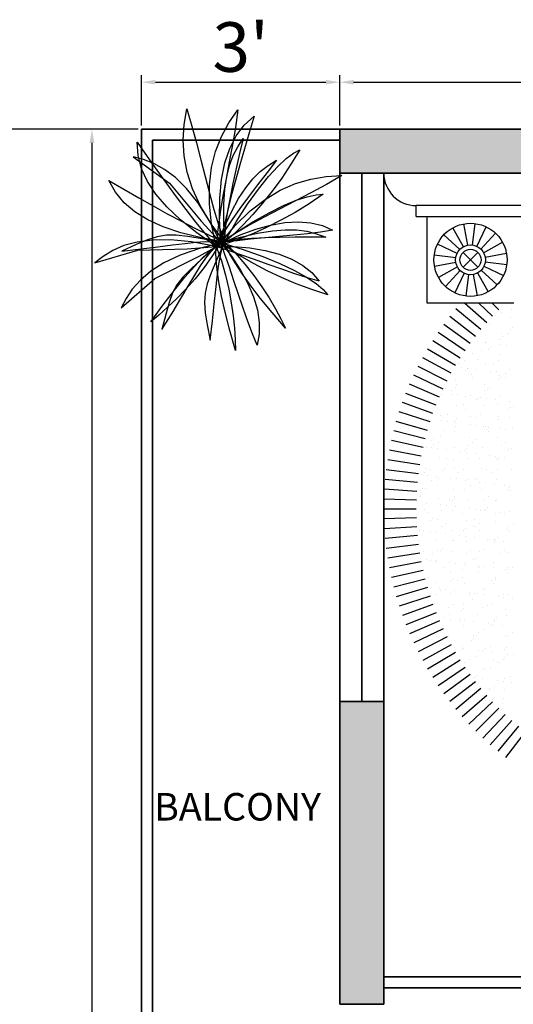
# Model space of a CAD drawing. Units: inches. Extents: x 1566 to 2546, y 1087 to 2705.
# Tile 20 of 27: x 2040 to 2130, y 1625 to 1804. Entities that reach past the tile are written whole.
import ezdxf

# ---------------------------------------------------------------- set-up
doc = ezdxf.new("R2010")
doc.units = ezdxf.units.IN
for name, color, linetype, lineweight in [('A-ANNO-DIMS', 2, 'Continuous', 18), ('A-AREA-IDEN', 7, 'Continuous', 18), ('A-FURN', 8, 'Continuous', 18), ('A-WALL', 7, 'Continuous', 35), ('A-WALL-PATT', 8, 'Continuous', 13), ('L-PLNT', 94, 'Continuous', 18)]:
    doc.layers.add(name, color=color, linetype=linetype, lineweight=lineweight)
for name, color, linetype in [('A-FRN', 11, 'Continuous'), ('A-HT', 15, 'Continuous'), ('DIENHOA', 3, 'Continuous'), ('L-HT', 1, 'Continuous')]:
    doc.layers.add(name, color=color, linetype=linetype)
doc.styles.get("Standard").update_dxf_attribs({"font": 'arial.ttf'})
doc.dimstyles.new('ISO-25', dxfattribs={"dimtxt": 2.5, "dimasz": 2.5, "dimexe": 1.25, "dimexo": 0.625, "dimtad": 1, "dimtxsty": 'Standard', "dimcen": 2.5, "dimadec": 0, "dimazin": 0, "dimtfac": 1, "dimtmove": 0, "dimatfit": 3, "dimfxl": 1, "dimarcsym": 0})

# ---------------------------------------------------------------- blocks, each defined once
blk = doc.blocks.new('*D1')
at = {"layer": 'A-ANNO-DIMS', "color": 0, "lineweight": -2, "transparency": 16777216}
for p, q in [((2062.29, 1785.06), (2062.29, 1794.2)), ((2098.29, 1785.06), (2098.29, 1794.2)), ((2064.79, 1792.95), (2095.79, 1792.95))]:
    blk.add_line(p, q, dxfattribs=at)
at = {"layer": 'A-ANNO-DIMS', "color": 0, "transparency": 16777216}
for points in [[(2064.79, 1793.37), (2064.79, 1792.53), (2062.29, 1792.95)], [(2095.79, 1793.37), (2095.79, 1792.53), (2098.29, 1792.95)]]:
    blk.add_solid(points, dxfattribs=at)
at = {"layer": 'Defpoints', "color": 0, "transparency": 16777216}
for p in [(2098.29, 1792.95), (2062.29, 1784.43), (2098.29, 1784.43)]:
    blk.add_point(p, dxfattribs=at)
at = {"layer": 'A-ANNO-DIMS', "color": 0, "transparency": 16777216, "insert": (2080.29, 1798.17), "char_height": 9, "attachment_point": 5}
blk.add_mtext("3'", dxfattribs=at)
blk = doc.blocks.new('*D2')
at = {"layer": 'A-ANNO-DIMS', "color": 0, "lineweight": -2, "transparency": 16777216}
for p, q in [((2098.29, 1785.06), (2098.29, 1794.2)), ((2458.29, 1785.06), (2458.29, 1794.2)), ((2100.79, 1792.95), (2455.79, 1792.95))]:
    blk.add_line(p, q, dxfattribs=at)
at = {"layer": 'A-ANNO-DIMS', "color": 0, "transparency": 16777216}
for points in [[(2100.79, 1793.37), (2100.79, 1792.53), (2098.29, 1792.95)], [(2455.79, 1793.37), (2455.79, 1792.53), (2458.29, 1792.95)]]:
    blk.add_solid(points, dxfattribs=at)
at = {"layer": 'Defpoints', "color": 0, "transparency": 16777216}
for p in [(2458.29, 1792.95), (2098.29, 1784.43), (2458.29, 1784.43)]:
    blk.add_point(p, dxfattribs=at)
at = {"layer": 'A-ANNO-DIMS', "color": 0, "transparency": 16777216, "insert": (2278.29, 1798.17), "char_height": 9, "attachment_point": 5}
blk.add_mtext("30'", dxfattribs=at)
blk = doc.blocks.new('*D3')
at = {"layer": 'A-ANNO-DIMS', "color": 0, "lineweight": -2, "transparency": 16777216}
for p, q in [((2061.66, 1784.43), (2052.02, 1784.43)), ((2053.27, 1781.93), (2053.27, 1162.93)), ((2061.66, 1160.43), (2052.02, 1160.43))]:
    blk.add_line(p, q, dxfattribs=at)
at = {"layer": 'A-ANNO-DIMS', "color": 0, "transparency": 16777216}
for points in [[(2052.85, 1781.93), (2053.69, 1781.93), (2053.27, 1784.43)], [(2052.85, 1162.93), (2053.69, 1162.93), (2053.27, 1160.43)]]:
    blk.add_solid(points, dxfattribs=at)
at = {"layer": 'Defpoints', "color": 0, "transparency": 16777216}
for p in [(2062.29, 1784.43), (2053.27, 1160.43), (2062.29, 1160.43)]:
    blk.add_point(p, dxfattribs=at)
at = {"layer": 'A-ANNO-DIMS', "color": 0, "transparency": 16777216, "insert": (2048.05, 1472.43), "char_height": 9, "attachment_point": 5, "rotation": 90}
blk.add_mtext("52'", dxfattribs=at)
blk = doc.blocks.new('*X21')
at = {"color": 0}
for p, q in [((1.0951, 2.4744), (1.0951, 2.4744)), ((1.0521, 2.4302), (1.0521, 2.4302)), ((1.0613, 2.4218), (1.0613, 2.4218)), ((1.0963, 2.4457), (1.0963, 2.4457)), ((1.1027, 2.4263), (1.1027, 2.4263)), ((1.0383, 2.3768), (1.0383, 2.3768)), ((1.0397, 2.3823), (1.0397, 2.3823)), ((1.0608, 2.3689), (1.0608, 2.3689)), ((1.1048, 2.3819), (1.1048, 2.3819)), ((0.966, 2.3279), (0.966, 2.3279)), ((0.9708, 2.3251), (0.9708, 2.3251)), ((0.981, 2.3202), (0.981, 2.3202)), ((1.0066, 2.3333), (1.0066, 2.3333)), ((1.0745, 2.3422), (1.0745, 2.3422)), ((1.1005, 2.3457), (1.1005, 2.3457)), ((1.1059, 2.33), (1.1059, 2.33)), ((1.1367, 2.3205), (1.1367, 2.3205)), ((1.1412, 2.351), (1.1412, 2.351)), ((1.0043, 2.2924), (1.0043, 2.2924)), ((1.0135, 2.284), (1.0135, 2.284)), ((1.0414, 2.2805), (1.0414, 2.2805)), ((0.9244, 2.2568), (0.9244, 2.2568)), ((0.9455, 2.2434), (0.9455, 2.2434)), ((0.974, 2.2287), (0.974, 2.2287)), ((1.057, 2.2441), (1.057, 2.2441)), ((1.0801, 2.2571), (1.0801, 2.2571)), ((1.1012, 2.2437), (1.1012, 2.2437)), ((1.109, 2.2336), (1.109, 2.2336)), ((0.8775, 2.1868), (0.8775, 2.1868)), ((0.9067, 2.2002), (0.9067, 2.2002)), ((0.9137, 2.1825), (0.9137, 2.1825)), ((0.9181, 2.1922), (0.9181, 2.1922)), ((0.986, 2.2011), (0.986, 2.2011)), ((1.0121, 2.2046), (1.0121, 2.2046)), ((1.0214, 2.195), (1.0214, 2.195)), ((1.0446, 2.1841), (1.0446, 2.1841)), ((1.0527, 2.2099), (1.0527, 2.2099)), ((1.1068, 2.1985), (1.1068, 2.1985)), ((1.116, 2.1901), (1.116, 2.1901)), ((1.1206, 2.2189), (1.1206, 2.2189)), ((1.1466, 2.2223), (1.1466, 2.2223)), ((0.9565, 2.1546), (0.9565, 2.1546)), ((0.9657, 2.1462), (0.9657, 2.1462)), ((1.1122, 2.1373), (1.1122, 2.1373)), ((0.8492, 2.133), (0.8492, 2.133)), ((0.9648, 2.1316), (0.9648, 2.1316)), ((0.9771, 2.1324), (0.9771, 2.1324)), ((0.9859, 2.1182), (0.9859, 2.1182)), ((1.0092, 2.1063), (1.0092, 2.1063)), ((1.1205, 2.1319), (1.1205, 2.1319)), ((1.1416, 2.1184), (1.1416, 2.1184)), ((0.8296, 2.0511), (0.8296, 2.0511)), ((0.8589, 2.0624), (0.8589, 2.0624)), ((0.8975, 2.06), (0.8975, 2.06)), ((0.9061, 2.0695), (0.9061, 2.0695)), ((0.9169, 2.0861), (0.9169, 2.0861)), ((0.9236, 2.0635), (0.9236, 2.0635)), ((0.9642, 2.0688), (0.9642, 2.0688)), ((1.0321, 2.0777), (1.0321, 2.0777)), ((1.0477, 2.0878), (1.0477, 2.0878)), ((1.0582, 2.0812), (1.0582, 2.0812)), ((1.059, 2.0607), (1.059, 2.0607)), ((1.0618, 2.0698), (1.0618, 2.0698)), ((1.0682, 2.0523), (1.0682, 2.0523)), ((1.0988, 2.0865), (1.0988, 2.0865)), ((0.8495, 2.0061), (0.8495, 2.0061)), ((0.8524, 2.0367), (0.8524, 2.0367)), ((0.9087, 2.0168), (0.9087, 2.0168)), ((0.9179, 2.0084), (0.9179, 2.0084)), ((0.9803, 2.0361), (0.9803, 2.0361)), ((1.0052, 2.0064), (1.0052, 2.0064)), ((1.1117, 2.0124), (1.1117, 2.0124)), ((1.1153, 2.0409), (1.1153, 2.0409)), ((0.785, 1.9849), (0.785, 1.9849)), ((0.8706, 1.9927), (0.8706, 1.9927)), ((0.92, 1.9898), (0.92, 1.9898)), ((0.9614, 1.9685), (0.9614, 1.9685)), ((1.0263, 1.993), (1.0263, 1.993)), ((1.0509, 1.9915), (1.0509, 1.9915)), ((1.0782, 1.9544), (1.0782, 1.9544)), ((1.1043, 1.9578), (1.1043, 1.9578)), ((1.1449, 1.9631), (1.1449, 1.9631)), ((0.7908, 1.944), (0.7908, 1.944)), ((0.8091, 1.9189), (0.8091, 1.9189)), ((0.8111, 1.9247), (0.8111, 1.9247)), ((0.8351, 1.9223), (0.8351, 1.9223)), ((0.8555, 1.9403), (0.8555, 1.9403)), ((0.8757, 1.9277), (0.8757, 1.9277)), ((0.9436, 1.9366), (0.9436, 1.9366)), ((0.9465, 1.9443), (0.9465, 1.9443)), ((0.9697, 1.9401), (0.9697, 1.9401)), ((0.9834, 1.9397), (0.9834, 1.9397)), ((1.0103, 1.9454), (1.0103, 1.9454)), ((1.0111, 1.9229), (1.0111, 1.9229)), ((1.0204, 1.9145), (1.0204, 1.9145)), ((1.1022, 1.9446), (1.1022, 1.9446)), ((1.1185, 1.9446), (1.1185, 1.9446)), ((0.7552, 1.8672), (0.7552, 1.8672)), ((0.7881, 1.8886), (0.7881, 1.8886)), ((0.8608, 1.879), (0.8608, 1.879)), ((0.8701, 1.8706), (0.8701, 1.8706)), ((0.8898, 1.8809), (0.8898, 1.8809)), ((0.9109, 1.8675), (0.9109, 1.8675)), ((0.9232, 1.8935), (0.9232, 1.8935)), ((1.0456, 1.8812), (1.0456, 1.8812)), ((1.054, 1.8951), (1.054, 1.8951)), ((1.0639, 1.8746), (1.0639, 1.8746)), ((1.0666, 1.8678), (1.0666, 1.8678)), ((0.8311, 1.8188), (0.8311, 1.8188)), ((0.8587, 1.844), (0.8587, 1.844)), ((0.9136, 1.8307), (0.9136, 1.8307)), ((0.9866, 1.8434), (0.9866, 1.8434)), ((0.9868, 1.8191), (0.9868, 1.8191)), ((1.0564, 1.822), (1.0564, 1.822)), ((1.1136, 1.829), (1.1136, 1.829)), ((1.1216, 1.8482), (1.1216, 1.8482)), ((1.1228, 1.8206), (1.1228, 1.8206)), ((1.1243, 1.831), (1.1243, 1.831)), ((1.1425, 1.8194), (1.1425, 1.8194)), ((0.7206, 1.7778), (0.7206, 1.7778)), ((0.7466, 1.7812), (0.7466, 1.7812)), ((0.7632, 1.7869), (0.7632, 1.7869)), ((0.7872, 1.7866), (0.7872, 1.7866)), ((0.7913, 1.7922), (0.7913, 1.7922)), ((0.8552, 1.7955), (0.8552, 1.7955)), ((0.8812, 1.799), (0.8812, 1.799)), ((0.9218, 1.8043), (0.9218, 1.8043)), ((0.9263, 1.7971), (0.9263, 1.7971)), ((0.9633, 1.7851), (0.9633, 1.7851)), ((0.9725, 1.7767), (0.9725, 1.7767)), ((0.9897, 1.8132), (0.9897, 1.8132)), ((1.0158, 1.8167), (1.0158, 1.8167)), ((1.0572, 1.7988), (1.0572, 1.7988)), ((0.731, 1.746), (0.731, 1.746)), ((0.7745, 1.7554), (0.7745, 1.7554)), ((0.7956, 1.742), (0.7956, 1.742)), ((0.813, 1.7413), (0.813, 1.7413)), ((0.8222, 1.7328), (0.8222, 1.7328)), ((0.8618, 1.7477), (0.8618, 1.7477)), ((0.9302, 1.7557), (0.9302, 1.7557)), ((0.9513, 1.7423), (0.9513, 1.7423)), ((0.9897, 1.747), (0.9897, 1.747)), ((1.016, 1.7368), (1.016, 1.7368)), ((1.0859, 1.756), (1.0859, 1.756)), ((1.107, 1.7426), (1.107, 1.7426)), ((1.1248, 1.7519), (1.1248, 1.7519)), ((0.7158, 1.6933), (0.7158, 1.6933)), ((0.7944, 1.6959), (0.7944, 1.6959)), ((0.8657, 1.693), (0.8657, 1.693)), ((0.8715, 1.6936), (0.8715, 1.6936)), ((0.9295, 1.7008), (0.9295, 1.7008)), ((1.0272, 1.6939), (1.0272, 1.6939)), ((1.0358, 1.6899), (1.0358, 1.6899)), ((1.0603, 1.7024), (1.0603, 1.7024)), ((1.0619, 1.6933), (1.0619, 1.6933)), ((1.0658, 1.6912), (1.0658, 1.6912)), ((1.075, 1.6828), (1.075, 1.6828)), ((1.1025, 1.6986), (1.1025, 1.6986)), ((0.7154, 1.6491), (0.7154, 1.6491)), ((0.7341, 1.6496), (0.7341, 1.6496)), ((0.7667, 1.6544), (0.7667, 1.6544)), ((0.7927, 1.6578), (0.7927, 1.6578)), ((0.8333, 1.6632), (0.8333, 1.6632)), ((0.865, 1.6513), (0.865, 1.6513)), ((0.9013, 1.6721), (0.9013, 1.6721)), ((0.9155, 1.6474), (0.9155, 1.6474)), ((0.9247, 1.6389), (0.9247, 1.6389)), ((0.9273, 1.6756), (0.9273, 1.6756)), ((0.9679, 1.6809), (0.9679, 1.6809)), ((0.9929, 1.6507), (0.9929, 1.6507)), ((1.1185, 1.6429), (1.1185, 1.6429)), ((1.1279, 1.6556), (1.1279, 1.6556)), ((0.7652, 1.6035), (0.7652, 1.6035)), ((0.7744, 1.595), (0.7744, 1.595)), ((0.7976, 1.5996), (0.7976, 1.5996)), ((0.8149, 1.6302), (0.8149, 1.6302)), ((0.836, 1.6168), (0.836, 1.6168)), ((0.9326, 1.6044), (0.9326, 1.6044)), ((0.9682, 1.599), (0.9682, 1.599)), ((0.9706, 1.6305), (0.9706, 1.6305)), ((0.9917, 1.6171), (0.9917, 1.6171)), ((1.0635, 1.6061), (1.0635, 1.6061)), ((1.1263, 1.6308), (1.1263, 1.6308)), ((1.1474, 1.6173), (1.1474, 1.6173)), ((0.7373, 1.5533), (0.7373, 1.5533)), ((0.7562, 1.5681), (0.7562, 1.5681)), ((0.8179, 1.5552), (0.8179, 1.5552)), ((0.8681, 1.555), (0.8681, 1.555)), ((0.9119, 1.5684), (0.9119, 1.5684)), ((0.9474, 1.5488), (0.9474, 1.5488)), ((0.9734, 1.5522), (0.9734, 1.5522)), ((0.996, 1.5544), (0.996, 1.5544)), ((1.014, 1.5575), (1.014, 1.5575)), ((1.018, 1.5534), (1.018, 1.5534)), ((1.0272, 1.545), (1.0272, 1.545)), ((1.0676, 1.5687), (1.0676, 1.5687)), ((1.0819, 1.5665), (1.0819, 1.5665)), ((1.108, 1.5699), (1.108, 1.5699)), ((1.1311, 1.5592), (1.1311, 1.5592)), ((0.7042, 1.5167), (0.7042, 1.5167)), ((0.7448, 1.5221), (0.7448, 1.5221)), ((0.8007, 1.5032), (0.8007, 1.5032)), ((0.8128, 1.531), (0.8128, 1.531)), ((0.8388, 1.5345), (0.8388, 1.5345)), ((0.8553, 1.505), (0.8553, 1.505)), ((0.8677, 1.5096), (0.8677, 1.5096)), ((0.8769, 1.5011), (0.8769, 1.5011)), ((0.8794, 1.5398), (0.8794, 1.5398)), ((0.9358, 1.5081), (0.9358, 1.5081)), ((1.011, 1.5053), (1.011, 1.5053)), ((1.0666, 1.5098), (1.0666, 1.5098)), ((1.0707, 1.5051), (1.0707, 1.5051)), ((0.7174, 1.4657), (0.7174, 1.4657)), ((0.7207, 1.4913), (0.7207, 1.4913)), ((0.7266, 1.4572), (0.7266, 1.4572)), ((0.7404, 1.457), (0.7404, 1.457)), ((0.8713, 1.4586), (0.8713, 1.4586)), ((0.8764, 1.4916), (0.8764, 1.4916)), ((0.9204, 1.4613), (0.9204, 1.4613)), ((0.9992, 1.458), (0.9992, 1.458)), ((1.0321, 1.4919), (1.0321, 1.4919)), ((1.1205, 1.4595), (1.1205, 1.4595)), ((1.1342, 1.4629), (1.1342, 1.4629)), ((0.7701, 1.4174), (0.7701, 1.4174)), ((0.7966, 1.4429), (0.7966, 1.4429)), ((0.8849, 1.4111), (0.8849, 1.4111)), ((0.9255, 1.4164), (0.9255, 1.4164)), ((0.9389, 1.4118), (0.9389, 1.4118)), ((0.9523, 1.4432), (0.9523, 1.4432)), ((0.9701, 1.4157), (0.9701, 1.4157)), ((0.9935, 1.4254), (0.9935, 1.4254)), ((1.0195, 1.4288), (1.0195, 1.4288)), ((1.0601, 1.4341), (1.0601, 1.4341)), ((1.0698, 1.4134), (1.0698, 1.4134)), ((1.108, 1.4435), (1.108, 1.4435)), ((1.128, 1.4431), (1.128, 1.4431)), ((1.1297, 1.4511), (1.1297, 1.4511)), ((0.7243, 1.3899), (0.7243, 1.3899)), ((0.74, 1.3795), (0.74, 1.3795)), ((0.7503, 1.3934), (0.7503, 1.3934)), ((0.761, 1.3661), (0.761, 1.3661)), ((0.7909, 1.3987), (0.7909, 1.3987)), ((0.8039, 1.4069), (0.8039, 1.4069)), ((0.8198, 1.3718), (0.8198, 1.3718)), ((0.8291, 1.3633), (0.8291, 1.3633)), ((0.8589, 1.4076), (0.8589, 1.4076)), ((0.8957, 1.3798), (0.8957, 1.3798)), ((0.9168, 1.3664), (0.9168, 1.3664)), ((0.9794, 1.4072), (0.9794, 1.4072)), ((1.0229, 1.3673), (1.0229, 1.3673)), ((1.0514, 1.3801), (1.0514, 1.3801)), ((1.0725, 1.3667), (1.0725, 1.3667)), ((1.1374, 1.3665), (1.1374, 1.3665)), ((0.7436, 1.3606), (0.7436, 1.3606)), ((0.837, 1.3177), (0.837, 1.3177)), ((0.8726, 1.3235), (0.8726, 1.3235)), ((0.8744, 1.3623), (0.8744, 1.3623)), ((0.9927, 1.318), (0.9927, 1.318)), ((1.0023, 1.3617), (1.0023, 1.3617)), ((1.0726, 1.3217), (1.0726, 1.3217)), ((0.807, 1.3105), (0.807, 1.3105)), ((0.837, 1.2753), (0.837, 1.2753)), ((0.905, 1.2843), (0.905, 1.2843)), ((0.9223, 1.2779), (0.9223, 1.2779)), ((0.931, 1.2877), (0.931, 1.2877)), ((0.9421, 1.3154), (0.9421, 1.3154)), ((0.9716, 1.293), (0.9716, 1.293)), ((1.0396, 1.302), (1.0396, 1.302)), ((1.0656, 1.3054), (1.0656, 1.3054)), ((1.0729, 1.3171), (1.0729, 1.3171)), ((1.0818, 1.3133), (1.0818, 1.3133)), ((1.1062, 1.3108), (1.1062, 1.3108)), ((1.1253, 1.2734), (1.1253, 1.2734)), ((0.7467, 1.2643), (0.7467, 1.2643)), ((0.7704, 1.2665), (0.7704, 1.2665)), ((0.772, 1.234), (0.772, 1.234)), ((0.7803, 1.2543), (0.7803, 1.2543)), ((0.7964, 1.27), (0.7964, 1.27)), ((0.8014, 1.2409), (0.8014, 1.2409)), ((0.8776, 1.2659), (0.8776, 1.2659)), ((0.9315, 1.2694), (0.9315, 1.2694)), ((0.936, 1.2546), (0.936, 1.2546)), ((0.9571, 1.2412), (0.9571, 1.2412)), ((0.975, 1.2296), (0.975, 1.2296)), ((1.0055, 1.2653), (1.0055, 1.2653)), ((1.0918, 1.2549), (1.0918, 1.2549)), ((1.1128, 1.2414), (1.1128, 1.2414)), ((1.1405, 1.2702), (1.1405, 1.2702)), ((0.7812, 1.2255), (0.7812, 1.2255)), ((0.8102, 1.2142), (0.8102, 1.2142)), ((0.8247, 1.1857), (0.8247, 1.1857)), ((0.8773, 1.1925), (0.8773, 1.1925)), ((0.9452, 1.2191), (0.9452, 1.2191)), ((1.0248, 1.184), (1.0248, 1.184)), ((1.033, 1.1928), (1.033, 1.1928)), ((1.0761, 1.2207), (1.0761, 1.2207)), ((1.1117, 1.182), (1.1117, 1.182)), ((0.8165, 1.1432), (0.8165, 1.1432)), ((0.8425, 1.1466), (0.8425, 1.1466)), ((0.8745, 1.1401), (0.8745, 1.1401)), ((0.8807, 1.1696), (0.8807, 1.1696)), ((0.8831, 1.1519), (0.8831, 1.1519)), ((0.9511, 1.1609), (0.9511, 1.1609)), ((0.9771, 1.1643), (0.9771, 1.1643)), ((1.0086, 1.169), (1.0086, 1.169)), ((1.0177, 1.1696), (1.0177, 1.1696)), ((1.034, 1.1755), (1.034, 1.1755)), ((1.0857, 1.1786), (1.0857, 1.1786)), ((1.1437, 1.1739), (1.1437, 1.1739)), ((0.8133, 1.1179), (0.8133, 1.1179)), ((0.8207, 1.1291), (0.8207, 1.1291)), ((0.8418, 1.1157), (0.8418, 1.1157)), ((0.8837, 1.1316), (0.8837, 1.1316)), ((0.9272, 1.0918), (0.9272, 1.0918)), ((0.9484, 1.1227), (0.9484, 1.1227)), ((0.9764, 1.1294), (0.9764, 1.1294)), ((0.9975, 1.116), (0.9975, 1.116)), ((1.0775, 1.1356), (1.0775, 1.1356)), ((1.0792, 1.1244), (1.0792, 1.1244)), ((1.1321, 1.1297), (1.1321, 1.1297)), ((0.8839, 1.0733), (0.8839, 1.0733)), ((0.9177, 1.0673), (0.9177, 1.0673)), ((0.977, 1.0462), (0.977, 1.0462)), ((1.0118, 1.0727), (1.0118, 1.0727)), ((1.0638, 1.0463), (1.0638, 1.0463)), ((1.0734, 1.0676), (1.0734, 1.0676)), ((1.1273, 1.09), (1.1273, 1.09)), ((1.1318, 1.0552), (1.1318, 1.0552)), ((1.1365, 1.0816), (1.1365, 1.0816)), ((1.1468, 1.0775), (1.1468, 1.0775)), ((0.8165, 1.0215), (0.8165, 1.0215)), ((0.8267, 1.0023), (0.8267, 1.0023)), ((0.8611, 1.0039), (0.8611, 1.0039)), ((0.8626, 1.0198), (0.8626, 1.0198)), ((0.8886, 1.0232), (0.8886, 1.0232)), ((0.9292, 1.0285), (0.9292, 1.0285)), ((0.9515, 1.0264), (0.9515, 1.0264)), ((0.9862, 1.0377), (0.9862, 1.0377)), ((0.9972, 1.0375), (0.9972, 1.0375)), ((1.0168, 1.0042), (1.0168, 1.0042)), ((1.0232, 1.0409), (1.0232, 1.0409)), ((1.0824, 1.0281), (1.0824, 1.0281)), ((0.8359, 0.9938), (0.8359, 0.9938)), ((0.8822, 0.9905), (0.8822, 0.9905)), ((0.887, 0.9769), (0.887, 0.9769)), ((1.0149, 0.9763), (1.0149, 0.9763)), ((1.0297, 0.9979), (1.0297, 0.9979)), ((1.0379, 0.9908), (1.0379, 0.9908)), ((0.8794, 0.954), (0.8794, 0.954)), ((0.9546, 0.93), (0.9546, 0.93)), ((0.9581, 0.9421), (0.9581, 0.9421)), ((1.0433, 0.9141), (1.0433, 0.9141)), ((1.0693, 0.9175), (1.0693, 0.9175)), ((1.0795, 0.9523), (1.0795, 0.9523)), ((1.0855, 0.9317), (1.0855, 0.9317)), ((1.0887, 0.9438), (1.0887, 0.9438)), ((1.1099, 0.9229), (1.1099, 0.9229)), ((1.1138, 0.9424), (1.1138, 0.9424)), ((0.8902, 0.8806), (0.8902, 0.8806)), ((0.9015, 0.8787), (0.9015, 0.8787)), ((0.9087, 0.8964), (0.9087, 0.8964)), ((0.9226, 0.8653), (0.9226, 0.8653)), ((0.9292, 0.9084), (0.9292, 0.9084)), ((0.9347, 0.8998), (0.9347, 0.8998)), ((0.9384, 0.8999), (0.9384, 0.8999)), ((0.9753, 0.9052), (0.9753, 0.9052)), ((1.0181, 0.88), (1.0181, 0.88)), ((1.0572, 0.879), (1.0572, 0.879)), ((1.0783, 0.8655), (1.0783, 0.8655)), ((1.1322, 0.904), (1.1322, 0.904)), ((0.9578, 0.8337), (0.9578, 0.8337)), ((0.9819, 0.8601), (0.9819, 0.8601)), ((1.0887, 0.8354), (1.0887, 0.8354)), ((0.9808, 0.7764), (0.9808, 0.7764)), ((0.9985, 0.8169), (0.9985, 0.8169)), ((1.0212, 0.7836), (1.0212, 0.7836)), ((1.0214, 0.7818), (1.0214, 0.7818)), ((1.0316, 0.8145), (1.0316, 0.8145)), ((1.0409, 0.806), (1.0409, 0.806)), ((1.0894, 0.7907), (1.0894, 0.7907)), ((1.1154, 0.7941), (1.1154, 0.7941)), ((1.0844, 0.7662), (1.0844, 0.7662)), ((1.0918, 0.739), (1.0918, 0.739)), ((1.0976, 0.7538), (1.0976, 0.7538)), ((1.1187, 0.7403), (1.1187, 0.7403)), ((1.0389, 0.6917), (1.0389, 0.6917)), ((1.1341, 0.7206), (1.1341, 0.7206)), ((1.1433, 0.7121), (1.1433, 0.7121)), ((1.0675, 0.6584), (1.0675, 0.6584)), ((1.095, 0.6427), (1.095, 0.6427)), ((1.1355, 0.6673), (1.1355, 0.6673)), ((1.138, 0.6286), (1.138, 0.6286))]:
    blk.add_line(p, q, dxfattribs=at)
blk = doc.blocks.new('A$C6796526C')
at = {"layer": 'A-FRN'}
for p, q in [((0, 3), (2.9, 3)), ((2.75, 2.85), (0.15, 2.85)), ((0.15, 2.8), (0.15, 2.85)), ((0.15, 2.8), (2.75, 2.8)), ((0.2, 2.4), (0.2, 2.8)), ((0.6, 2.4), (0.2, 2.4))]:
    blk.add_line(p, q, dxfattribs=at)
for radius in [0.1686, 0.0686]:
    blk.add_circle((0.4, 2.6), radius, dxfattribs=at)
blk.add_arc((0.15, 3), 0.15, 180, 270, dxfattribs=at)
at = {"layer": 'A-HT'}
for p, q in [((0.4483, 2.2787), (0.3328, 2.3743)), ((0.4749, 2.3097), (0.3724, 2.4)), ((0.5023, 2.3399), (0.4384, 2.4)), ((0.5308, 2.3692), (0.5, 2.4)), ((0.4228, 2.2468), (0.3043, 2.3387)), ((0.3983, 2.2141), (0.2769, 2.3023)), ((0.3524, 2.1466), (0.2257, 2.2269)), ((0.3748, 2.1807), (0.2507, 2.265)), ((0.331, 2.1118), (0.2019, 2.1881)), ((0.3108, 2.0763), (0.1794, 2.1485)), ((0.2917, 2.0402), (0.158, 2.1083)), ((0.2737, 2.0035), (0.138, 2.0674)), ((0.2569, 1.9663), (0.1193, 2.0259)), ((0.2413, 1.9286), (0.1018, 1.9838)), ((0.2269, 1.8904), (0.0857, 1.9412)), ((0.2136, 1.8517), (0.071, 1.8981)), ((0.2016, 1.8127), (0.0576, 1.8545)), ((0.1908, 1.7733), (0.0456, 1.8106)), ((0.1813, 1.7336), (0.0349, 1.7663)), ((0.173, 1.6936), (0.0257, 1.7217)), ((0.166, 1.6534), (0.0179, 1.6768)), ((0.1603, 1.6129), (0.0114, 1.6317)), ((0.1558, 1.5723), (0.0064, 1.5865)), ((0.1526, 1.5316), (0.0029, 1.541)), ((0.1506, 1.4908), (0.0007, 1.4955)), ((0.15, 1.45), (0, 1.45)), ((0.1506, 1.4092), (0.0007, 1.4045)), ((0.1526, 1.3684), (0.0029, 1.359)), ((0.1558, 1.3277), (0.0064, 1.3135)), ((0.1603, 1.2871), (0.0114, 1.2683)), ((0.166, 1.2466), (0.0179, 1.2232)), ((0.173, 1.2064), (0.0257, 1.1783)), ((0.1813, 1.1664), (0.0349, 1.1337)), ((0.1908, 1.1267), (0.0456, 1.0894)), ((0.2016, 1.0873), (0.0576, 1.0455)), ((0.2136, 1.0483), (0.071, 1.0019)), ((0.2269, 1.0096), (0.0857, 0.9588)), ((0.2413, 0.9714), (0.1018, 0.9162)), ((0.2569, 0.9337), (0.1193, 0.8741)), ((0.2737, 0.8965), (0.138, 0.8326)), ((0.2917, 0.8598), (0.158, 0.7917)), ((0.3108, 0.8237), (0.1794, 0.7515)), ((0.331, 0.7882), (0.2019, 0.7119)), ((0.3524, 0.7534), (0.2257, 0.6731)), ((0.3748, 0.7193), (0.2507, 0.635)), ((0.3983, 0.6859), (0.2769, 0.5977)), ((0.4228, 0.6532), (0.3043, 0.5613)), ((0.4483, 0.6213), (0.3328, 0.5257)), ((0.4749, 0.5903), (0.3623, 0.4911)), ((0.5023, 0.5601), (0.393, 0.4574)), ((0.5308, 0.5308), (0.4247, 0.4247)), ((0.5601, 0.5023), (0.4574, 0.393)), ((0.5903, 0.4749), (0.4911, 0.3623)), ((0.6213, 0.4483), (0.5257, 0.3328)), ((0.6532, 0.4228), (0.5613, 0.3043))]:
    blk.add_line(p, q, dxfattribs=at)
at = {"layer": 'L-HT'}
for p, q in [((0.3671, 2.6601), (0.319, 2.7478)), ((0.3873, 2.6674), (0.3687, 2.7656)), ((0.4087, 2.668), (0.4214, 2.7672)), ((0.4293, 2.662), (0.472, 2.7524)), ((0.3501, 2.647), (0.2773, 2.7156)), ((0.447, 2.6499), (0.5156, 2.7227)), ((0.4601, 2.6329), (0.5478, 2.681)), ((0.338, 2.6293), (0.2476, 2.672)), ((0.332, 2.6087), (0.2328, 2.6214)), ((0.3657, 2.5657), (0.4343, 2.6343)), ((0.4343, 2.5657), (0.3657, 2.6343)), ((0.4674, 2.6127), (0.5656, 2.6313)), ((0.468, 2.5913), (0.5672, 2.5786)), ((0.3326, 2.5873), (0.2344, 2.5687)), ((0.3399, 2.5671), (0.2522, 2.519)), ((0.353, 2.5501), (0.2844, 2.4773)), ((0.4499, 2.553), (0.5227, 2.4844)), ((0.462, 2.5707), (0.5524, 2.528)), ((0.3707, 2.538), (0.328, 2.4476)), ((0.3913, 2.532), (0.3786, 2.4328)), ((0.4127, 2.5326), (0.4313, 2.4344)), ((0.4329, 2.5399), (0.481, 2.4522))]:
    blk.add_line(p, q, dxfattribs=at)
blk.add_circle((0.4, 2.6), 0.0486, dxfattribs=at)
at = {"layer": 'A-HT', "extrusion": (0, 0, -1), "zscale": -1, "rotation": 180}
blk.add_blockref('*X21', (0.55, 3), dxfattribs=at)
blk = doc.blocks.new('Cay03_mb')
at = {"layer": 'DIENHOA'}
for p, q in [((118.6, 555.3), (166.2, 599.1)), ((166.2, 599.1), (142.2, 519.4)), ((79.5, 503.7), (118.6, 555.3)), ((142.2, 519.4), (119, 441.7)), ((48.6, 443.6), (79.5, 503.7)), ((25.5, 374.3), (48.6, 443.6)), ((119, 441.7), (96.7, 365.6)), ((-365.2, 390.3), (-414.4, 402.8)), ((-414.4, 402.8), (-240.2, 277.8)), ((-314.9, 371.3), (-365.2, 390.3)), ((-263.5, 343.5), (-314.9, 371.3)), ((-211.2, 304.6), (-263.5, 343.5)), ((9.9, 295.3), (25.5, 374.3)), ((96.7, 365.6), (75.6, 290.6)), ((-158, 252.3), (-211.2, 304.6)), ((1.6, 205.7), (9.9, 295.3)), ((75.6, 290.6), (55.7, 216.3)), ((363.4, 275.4), (436.8, 297.2)), ((436.8, 297.2), (511, 309.6)), ((511, 309.6), (585.9, 313.5)), ((585.9, 313.5), (511.8, 271.4)), ((-240.2, 277.8), (-88.4, 94.9)), ((-104.2, 184.4), (-158, 252.3)), ((218.5, 199.8), (290.6, 243.2)), ((290.6, 243.2), (363.4, 275.4)), ((511.8, 271.4), (437.6, 231.5)), ((0.2, 104.9), (1.6, 205.7)), ((55.7, 216.3), (37.3, 142.1)), ((147, 144.1), (218.5, 199.8)), ((363.7, 192.9), (290.2, 154.9)), ((437.6, 231.5), (363.7, 192.9)), ((-49.6, 98.5), (-104.2, 184.4)), ((37.3, 142.1), (20.5, 67.6)), ((75.9, 75.2), (147, 144.1)), ((290.2, 154.9), (217.4, 116.6)), ((-88.4, 94.9), (5.4, -7.8)), ((5.4, -7.8), (-49.6, 98.5)), ((5.4, -7.8), (0.2, 104.9)), ((217.4, 116.6), (145.5, 77.3)), ((5.4, -7.8), (75.9, 75.2)), ((20.5, 67.6), (5.4, -7.8)), ((145.5, 77.3), (74.7, 36.1)), ((182.2, 37.2), (253, 48.9)), ((253, 48.9), (314.6, 54.1)), ((314.6, 54.1), (369.2, 53.3)), ((369.2, 53.3), (418.6, 46.8)), ((-345, 5.4), (-399.6, -17.1)), ((-298.6, 20.1), (-345, 5.4)), ((-254.7, 27.4), (-298.6, 20.1)), ((-208, 27.8), (-254.7, 27.4)), ((-152.7, 21.7), (-208, 27.8)), ((-83.4, 9.7), (-152.7, 21.7)), ((5.4, -7.8), (-83.4, 9.7)), ((74.7, 36.1), (5.4, -7.8)), ((5.4, -7.8), (100.3, 18.4)), ((46.3, 0.9), (5.4, -7.8)), ((96.7, 7.5), (46.3, 0.9)), ((155, 12.2), (96.7, 7.5)), ((100.3, 18.4), (182.2, 37.2)), ((219.6, 15.4), (155, 12.2)), ((289, 17.4), (219.6, 15.4)), ((361.6, 18.5), (289, 17.4)), ((435.8, 18.9), (361.6, 18.5)), ((418.6, 46.8), (464.9, 35.2)), ((510, 19), (435.8, 18.9)), ((464.9, 35.2), (510, 19)), ((-399.6, -17.1), (-468, -47.9)), ((-468, -47.9), (-375.6, -37.8)), ((-375.6, -37.8), (-295.3, -27.9)), ((-295.3, -27.9), (-225.8, -18.9)), ((-225.8, -18.9), (-165.8, -11.3)), ((-165.8, -11.3), (-114, -5.7)), ((-114, -5.7), (-69, -2.9)), ((-79.8, -79.6), (-45.1, -46.3)), ((-69, -2.9), (-29.6, -3.4)), ((-45.1, -46.3), (-16.5, -22.4)), ((5.4, -7.8), (-33.2, -69.5)), ((-29.6, -3.4), (5.4, -7.8)), ((-16.5, -22.4), (5.4, -7.8)), ((5.4, -7.8), (56.8, -73.3)), ((25.9, -64.4), (5.4, -7.8)), ((5.4, -7.8), (112.8, -40.3)), ((53.5, -41.6), (5.4, -7.8)), ((107, -75.7), (53.5, -41.6)), ((112.8, -40.3), (207.5, -73.8)), ((-120.2, -122.1), (-79.8, -79.6)), ((-33.2, -69.5), (-74.6, -127.3)), ((47, -125.9), (25.9, -64.4)), ((56.8, -73.3), (100.4, -139.1)), ((165.5, -109.6), (107, -75.7)), ((207.5, -73.8), (289.5, -107.6)), ((-165.9, -174.1), (-120.2, -122.1)), ((-74.6, -127.3), (-117.8, -181.1)), ((68.7, -190.6), (47, -125.9)), ((100.4, -139.1), (135.9, -204.3)), ((228.7, -142.8), (165.5, -109.6)), ((289.5, -107.6), (359.3, -141.1)), ((359.3, -141.1), (416.9, -173.5)), ((-216.3, -235.6), (-165.9, -174.1)), ((-117.8, -181.1), (-162.1, -230.9)), ((296, -174.7), (228.7, -142.8)), ((367.1, -204.8), (296, -174.7)), ((416.9, -173.5), (462.6, -204.2)), ((-271, -306.6), (-216.3, -235.6)), ((-162.1, -230.9), (-206.3, -276.5)), ((90.8, -256.6), (68.7, -190.6)), ((135.9, -204.3), (162.8, -268.3)), ((441.6, -232.7), (367.1, -204.8)), ((518.9, -257.7), (441.6, -232.7)), ((462.6, -204.2), (496.5, -232.5)), ((496.5, -232.5), (518.9, -257.7)), ((-206.3, -276.5), (-249.6, -317.8)), ((113.1, -322.2), (90.8, -256.6)), ((162.8, -268.3), (181, -330.4)), ((-329.5, -387.1), (-271, -306.6)), ((-249.6, -317.8), (-291, -354.7)), ((135.4, -385.6), (113.1, -322.2)), ((181, -330.4), (190, -390)), ((-291, -354.7), (-329.5, -387.1)), ((157.6, -445), (135.4, -385.6)), ((190, -390), (189.6, -446.3)), ((179.5, -498.7), (157.6, -445)), ((189.6, -446.3), (179.5, -498.7))]:
    blk.add_line(p, q, dxfattribs=at)
for points in [[(23.7, -5.4), (-41, 82.2), (-91.8, 167.1), (-129.7, 249.5), (-155.6, 329.6), (-170.2, 407.8), (-174.7, 484.2), (-169.8, 559.3), (-156.5, 633.1)], [(-156.5, 633.1), (-132.5, 551.3), (-110.5, 470), (-89.8, 389.2), (-69.6, 309), (-49, 229.4), (-27.1, 150.4), (-3.2, 72.1), (23.7, -5.4)], [(-16.4, -26.7), (-38.3, 80), (-48.9, 178.3), (-48.7, 269), (-38.5, 352.6), (-19.1, 429.7), (9, 501), (44.9, 567.1), (87.9, 628.5)], [(87.9, 628.5), (75.5, 544.2), (61.3, 461.2), (46.1, 379.1), (30.8, 297.8), (16.1, 216.9), (2.9, 136), (-8.3, 54.9), (-16.4, -26.7)], [(-395.6, 473.7), (-347.5, 405.6), (-300.6, 339.5), (-254.3, 275.1), (-208.3, 212.3), (-161.9, 150.9), (-114.8, 90.7), (-66.5, 31.6), (-16.4, -26.7)], [(-16.4, -26.7), (-108.3, 38.6), (-186.9, 101.7), (-252.4, 163.5), (-305.1, 224.4), (-345.4, 285.2), (-373.7, 346.6), (-390.4, 409.2), (-395.6, 473.7)], [(23.7, -5.4), (19.8, 93), (20.3, 177), (25, 248.5), (34, 309.8), (47.3, 362.7), (64.9, 409.3), (86.8, 451.7), (112.9, 491.9)], [(112.9, 491.9), (96, 419.7), (79.5, 347.4), (63.9, 276.5), (50, 208.4), (38.4, 144.8), (29.7, 86.9), (24.6, 36.3), (23.7, -5.4)], [(384.3, 437.5), (342.2, 367.8), (298.1, 301.7), (252.6, 239.4), (206.1, 181.1), (159.4, 127.2), (113, 78), (67.6, 33.6), (23.7, -5.4)], [(23.7, -5.4), (79.9, 91.7), (134.1, 176.2), (185.8, 248.4), (234.3, 308.7), (279, 357.3), (319.3, 394.8), (354.6, 421.4), (384.3, 437.5)], [(273.2, 387.3), (227.6, 328.8), (182.3, 270.1), (138.4, 212.3), (97.2, 156.4), (60, 103.4), (27.8, 54.6), (1.9, 10.8), (-16.4, -26.7)], [(-16.4, -26.7), (21.4, 64.2), (57, 140.3), (91.4, 203.3), (125.2, 255.1), (159.5, 297.5), (195, 332.5), (232.7, 361.8), (273.2, 387.3)], [(-530.5, 289.7), (-458.3, 248.1), (-387.9, 207.8), (-318.9, 168.7), (-250.8, 131.1), (-182.9, 94.8), (-114.9, 59.9), (-46.2, 26.5), (23.7, -5.4)], [(23.7, -5.4), (-87.2, 15.2), (-185, 39.6), (-270.3, 68.2), (-343.7, 101.4), (-405.9, 139.7), (-457.3, 183.5), (-498.7, 233.4), (-530.5, 289.7)], [(496.7, 224), (429.4, 178.4), (361.6, 136.9), (294.1, 99.5), (227.5, 66.1), (162.4, 36.7), (99.7, 11.5), (39.8, -9.7), (-16.4, -26.7)], [(-16.4, -26.7), (75.4, 37.9), (160.1, 91.8), (237.3, 135.7), (306.6, 170), (367.6, 195.4), (419.9, 212.5), (463.1, 221.9), (496.7, 224)], [(23.7, -5.4), (99.3, 29.7), (173.2, 57.1), (244.8, 76.7), (313.3, 88.3), (377.9, 91.8), (437.9, 87), (492.7, 73.8), (541.4, 52)], [(541.4, 52), (484.1, 42.9), (421.2, 34.8), (354.4, 27.6), (285.4, 20.9), (216.1, 14.5), (148.2, 8.1), (83.5, 1.6), (23.7, -5.4)], [(-16.4, -26.7), (-134, -4.7), (-235.3, 5.3), (-322, 4.7), (-395.9, -5), (-458.7, -22.3), (-512.3, -45.7), (-558.2, -73.6), (-598.4, -104.7)], [(-598.4, -104.7), (-392.7, -44.4), (-155, -37.4), (-16.4, -26.7)], [(-471.9, -320.3), (-310.5, -179.3), (-97.7, -73.3), (23.7, -5.4)], [(23.7, -5.4), (-92.3, -34.8), (-188.4, -68.2), (-266.9, -105.1), (-329.9, -144.9), (-379.7, -187), (-418.5, -230.7), (-448.5, -275.3), (-471.9, -320.3)], [(-276.2, -424.4), (-227.3, -345.4), (-185.7, -276.1), (-150, -215.7), (-119.1, -163.8), (-91.5, -119.5), (-66, -82.3), (-41.4, -51.6), (-16.4, -26.7)], [(-16.4, -26.7), (-84.9, -86), (-137, -133.1), (-175.8, -173), (-204.3, -210), (-225.5, -249.1), (-242.5, -294.7), (-258.4, -351.6), (-276.2, -424.4)], [(23.7, -5.4), (-13.6, -87.9), (-41.1, -152.6), (-59.6, -205), (-69.9, -250.7), (-72.8, -295), (-69.2, -343.6), (-59.7, -401.9), (-45.3, -475.5)], [(-45.3, -475.5), (-34.1, -383.2), (-25.4, -302.8), (-18.3, -233.1), (-12, -172.9), (-5.6, -121.2), (2, -76.8), (11.4, -38.5), (23.7, -5.4)], [(76.2, -524.2), (48.8, -428.5), (26.6, -341.7), (9.2, -264.1), (-3.6, -196.1), (-12.3, -138), (-17.1, -90.2), (-18.3, -53), (-16.4, -26.7)], [(-16.4, -26.7), (66.9, -26.6), (145.6, -32.7), (218.8, -44.9), (285.8, -63.1), (345.9, -87.1), (398.4, -116.6), (442.6, -151.6), (477.6, -191.8)], [(477.6, -191.8), (421.8, -176), (361.3, -156.9), (297.6, -135.5), (232.2, -112.6), (166.6, -89.4), (102.3, -66.6), (40.8, -45.4), (-16.4, -26.7)], [(-16.4, -26.7), (8.5, -95.1), (28.5, -163.3), (44.3, -230.6), (56.3, -296.1), (65, -359), (70.9, -418.5), (74.5, -473.9), (76.2, -524.2)], [(316.5, -418.1), (251.4, -342.8), (194.8, -273.3), (146.5, -210.2), (106.3, -153.8), (74.1, -104.7), (49.7, -63.4), (32.9, -30.1), (23.7, -5.4)], [(23.7, -5.4), (74.9, -57.1), (121.8, -110.6), (164.3, -165), (202.7, -219.4), (237, -272.9), (267.3, -324.5), (293.7, -373.2), (316.5, -418.1)]]:
    blk.add_lwpolyline(points, dxfattribs=at)
blk = doc.blocks.new('*D91')
at = {"layer": 'A-ANNO-DIMS', "color": 0, "lineweight": -2, "transparency": 16777216}
for p, q in [((2061.66, 1784.43), (2016.94, 1784.43)), ((2018.19, 1781.93), (2018.19, 1531.18)), ((2061.66, 1528.68), (2016.94, 1528.68))]:
    blk.add_line(p, q, dxfattribs=at)
at = {"layer": 'A-ANNO-DIMS', "color": 0, "transparency": 16777216}
for points in [[(2017.77, 1781.93), (2018.6, 1781.93), (2018.19, 1784.43)], [(2017.77, 1531.18), (2018.6, 1531.18), (2018.19, 1528.68)]]:
    blk.add_solid(points, dxfattribs=at)
at = {"layer": 'Defpoints', "color": 0, "transparency": 16777216}
for p in [(2062.29, 1784.43), (2018.19, 1528.68), (2062.29, 1528.68)]:
    blk.add_point(p, dxfattribs=at)
at = {"layer": 'A-ANNO-DIMS', "color": 0, "transparency": 16777216, "insert": (2016.31, 1656.56), "char_height": 2.5, "attachment_point": 5, "rotation": 90}
blk.add_mtext('21\'-4"', dxfattribs=at)

msp = doc.modelspace()

# ---------------------------------------------------------------- hatches: boundary and pattern name
at = {"layer": 'A-WALL-PATT'}
h = msp.add_hatch(color=256, dxfattribs=at)
h.dxf.hatch_style = 1
h.paths.add_polyline_path([(2106.29, 1385.43), (2228.29, 1385.43), (2228.29, 1391.43), (2224.29, 1391.43), (2224.29, 1389.43), (2106.29, 1389.43), (2106.29, 1402.93), (2098.29, 1402.93), (2098.29, 1343.43), (2106.29, 1343.43), (2106.29, 1347.74)], flags=17)
h.paths.add_polyline_path([(2106.29, 1259.43), (2098.29, 1259.43), (2098.29, 1209.43), (2155.29, 1209.43), (2155.29, 1217.43), (2143.41, 1217.43), (2106.29, 1217.43)], flags=17)
h.paths.add_polyline_path([(2334.29, 1217.43), (2280.29, 1217.43), (2280.29, 1389.43), (2284.29, 1389.43), (2284.29, 1391.43), (2284.29, 1393.43), (2276.29, 1393.43), (2276.29, 1217.43), (2227.29, 1217.43), (2227.29, 1209.43), (2334.29, 1209.43)], flags=17)
h.paths.add_polyline_path([(2106.29, 1486.43), (2098.29, 1486.43), (2098.29, 1460.88), (2099.11, 1461.64), (2100.44, 1462.65), (2101.57, 1463.26), (2099.97, 1460.62), (2098.29, 1458.1), (2098.29, 1456.93), (2100.35, 1456.93), (2100.77, 1457.12), (2103.56, 1457.95), (2106.29, 1458.4), (2106.29, 1470.43), (2224.29, 1470.43), (2224.29, 1427.43), (2228.29, 1427.43), (2228.29, 1474.43), (2192.29, 1474.43), (2192.29, 1476.43), (2188.29, 1476.43), (2188.29, 1474.43), (2106.29, 1474.43)], flags=17)
h.paths.add_polyline_path([(2106.29, 1585.43), (2192.29, 1585.43), (2192.29, 1589.43), (2098.29, 1589.43), (2098.29, 1573.93), (2106.29, 1573.93)], flags=17)
h.paths.add_polyline_path([(2228.29, 1585.43), (2232.29, 1585.43), (2232.29, 1589.43), (2224.29, 1589.43), (2222.29, 1589.43), (2222.29, 1585.43), (2224.29, 1585.43), (2224.29, 1532.43), (2106.29, 1532.43), (2106.29, 1543.93), (2098.29, 1543.93), (2098.29, 1516.43), (2106.29, 1516.43), (2106.29, 1528.43), (2188.29, 1528.43), (2188.29, 1506.43), (2192.29, 1506.43), (2192.29, 1528.43), (2224.29, 1528.43), (2224.29, 1506.43), (2228.29, 1506.43)], flags=17)
h.paths.add_polyline_path([(2106.29, 1680.43), (2098.29, 1680.43), (2098.29, 1625.43), (2106.29, 1625.43)], flags=17)
h.paths.add_polyline_path([(2458.29, 1784.43), (2098.29, 1784.43), (2098.29, 1776.43), (2276.29, 1776.43), (2276.29, 1589.43), (2268.29, 1589.43), (2268.29, 1585.43), (2280.29, 1585.43), (2280.29, 1652.43), (2284.29, 1652.43), (2284.29, 1656.43), (2280.29, 1656.43), (2280.29, 1776.43), (2398.29, 1776.43), (2398.29, 1746.43), (2402.29, 1746.43), (2402.29, 1776.43), (2450.29, 1776.43), (2450.29, 1532.43), (2375.49, 1532.43), (2328.29, 1532.43), (2328.29, 1612.43), (2324.29, 1612.43), (2324.29, 1528.43), (2450.29, 1528.43), (2450.29, 1447.43), (2291.29, 1447.43), (2291.29, 1443.43), (2324.29, 1443.43), (2324.29, 1393.43), (2320.29, 1393.43), (2320.29, 1389.43), (2330.29, 1389.43), (2330.29, 1393.43), (2328.29, 1393.43), (2328.29, 1443.43), (2412.29, 1443.43), (2412.29, 1433.43), (2416.29, 1433.43), (2416.29, 1443.43), (2450.29, 1443.43), (2450.29, 1393.43), (2416.29, 1393.43), (2416.29, 1403.43), (2412.29, 1403.43), (2412.29, 1393.43), (2360.29, 1393.43), (2360.29, 1389.43), (2450.29, 1389.43), (2450.29, 1217.43), (2396.29, 1217.43), (2396.29, 1209.43), (2450.29, 1209.43), (2450.29, 1136.43), (2458.29, 1136.43)])

# ---------------------------------------------------------------- linework, layer by layer
at = {"layer": 'A-WALL'}
for p, q in [((2062.29, 1528.68), (2062.29, 1784.43)), ((2062.29, 1784.43), (2098.29, 1784.43)), ((2098.29, 1784.43), (2458.29, 1784.43)), ((2098.29, 1625.43), (2098.29, 1784.43)), ((2064.29, 1530.68), (2064.29, 1782.43)), ((2064.29, 1782.43), (2098.29, 1782.43)), ((2098.29, 1776.43), (2276.29, 1776.43)), ((2102.29, 1680.43), (2102.29, 1776.43)), ((2106.29, 1625.43), (2106.29, 1776.43)), ((2098.29, 1680.43), (2106.29, 1680.43)), ((2106.29, 1630.43), (2202.29, 1630.43)), ((2106.29, 1628.43), (2202.29, 1628.43)), ((2098.29, 1625.43), (2106.29, 1625.43))]:
    msp.add_line(p, q, dxfattribs=at)

# ---------------------------------------------------------------- block references
at = {"layer": 'A-FURN', "xscale": 39.3701, "yscale": 39.3701, "zscale": 39.3701}
msp.add_blockref('A$C6796526C', (2106.29, 1658.32), dxfattribs=at)
at = {"layer": 'L-PLNT', "xscale": 0.0378941924884598, "yscale": 0.0378941924884598, "zscale": 0.0378941924884598}
msp.add_blockref('Cay03_mb', (2076.46, 1764.1), dxfattribs=at)

# ---------------------------------------------------------------- texts
at = {"layer": 'A-AREA-IDEN', "insert": (2064.58, 1663.82), "char_height": 5, "attachment_point": 1}
msp.add_mtext_dynamic_manual_height_columns('BALCONY', width=111.7553, gutter_width=12.5, heights=[0], dxfattribs=at)

# ---------------------------------------------------------------- dimensions: what is measured, and where the dimension line sits
at = {"layer": 'A-ANNO-DIMS'}
for base, p1, p2, override, picture, middle in [((2098.29, 1792.95), (2062.29, 1784.43), (2098.29, 1784.43), {"dimtxt": 9, "dimdec": 1, "dimlunit": 3, "dimclrd": 0, "dimclre": 0, "dimclrt": 0, "dimtdec": 1}, '*D1', (2080.29, 1798.17)), ((2458.29, 1792.95), (2098.29, 1784.43), (2458.29, 1784.43), {"dimtxt": 9, "dimdec": 1, "dimlunit": 3, "dimclrd": 0, "dimclre": 0, "dimclrt": 0, "dimtdec": 1, "dimtmove": 1}, '*D2', (2278.29, 1798.17))]:
    dim = msp.add_linear_dim(base=base, p1=p1, p2=p2, dimstyle='ISO-25', override=override, dxfattribs=at)
    dim.commit()
    dim.dimension.update_dxf_attribs({"geometry": picture, "text_midpoint": middle})
for base, p1, p2, override, picture, middle in [((2018.1868, 1528.6802), (2062.2895, 1784.433), (2062.2895, 1528.6802), {"dimdec": 1, "dimlfac": 1, "dimrnd": 0, "dimzin": 1, "dimdsep": 46, "dimlunit": 4, "dimfrac": 2}, '*D91', (2016.3067, 1656.5566)), ((2053.27, 1160.43), (2062.29, 1784.43), (2062.29, 1160.43), {"dimtxt": 9, "dimdec": 1, "dimlunit": 3, "dimclrd": 0, "dimclre": 0, "dimclrt": 0, "dimtdec": 1}, '*D3', (2048.05, 1472.43))]:
    dim = msp.add_linear_dim(base=base, p1=p1, p2=p2, angle=90, dimstyle='ISO-25', override=override, dxfattribs=at)
    dim.commit()
    dim.dimension.update_dxf_attribs({"geometry": picture, "text_midpoint": middle})

doc.saveas('drawing.dxf')
